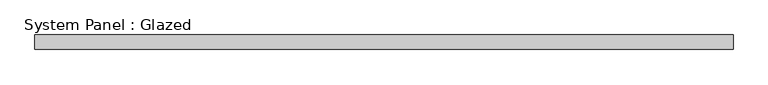
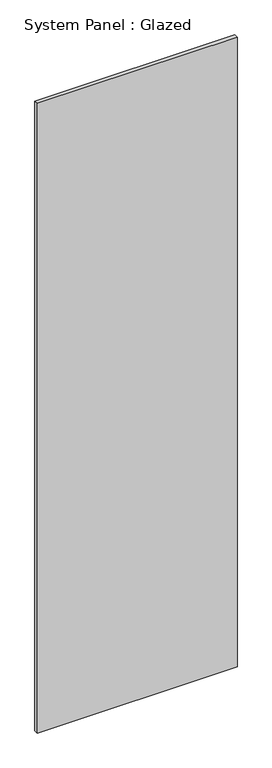
"""IFC4 building model written with IfcOpenShell, lengths in millimetres: plate geometry, System Panel : Glazed."""

from ifc_helpers import new_model, si_unit, origin, origin_with_axes, place, context, project, spatial, polyline, outline, extrude, source, transform, mapped, element, save


def system_panel_glazed_3e513c0f(model_context):
    return source(origin(), model_context, "Body", "SweptSolid", [
        extrude(outline(polyline([(600.1004, 24.5), (-600.1004, 24.5), (-600.1004, 49.5), (600.1004, 49.5), (600.1004, 24.5)])), origin_with_axes(), (0.0, 0.0, 1.0), 4000.0),
    ])


if __name__ == "__main__":
    model = new_model("IFC4")
    model_context = context("Model", 3, world=origin())
    ifc_project = project(units=[si_unit("LENGTHUNIT", "METRE", prefix="MILLI")], contexts=[model_context])
    site = spatial("IfcSite", under=ifc_project)
    building = spatial("IfcBuilding", under=site)
    placement = place(None, origin())
    system_panel_glazed_shape = system_panel_glazed_3e513c0f(model_context)
    element("IfcPlate", 1, ObjectType="System Panel : Glazed", at=placement, inside=building, context=model_context, shape_type="MappedRepresentation", body=[
        mapped(system_panel_glazed_shape, transform((0.0, 0.0, 0.0), x_axis=(1.0, 0.0, 0.0), y_axis=(0.0, 1.0, 0.0), z_axis=(0.0, 0.0, 1.0))),
    ])
    save(model, "model.ifc")

# Revit data of these elements
# Type "System Panel : Glazed"
#   Keynote = "H11"
#   Construction Type Id = "GSP4R"
#   Analytic Construction = "1/8 in Pilkington single glazing"
#   Visual Light Transmittance = 0.9
#   Solar Heat Gain Coefficient = 0.86
#   Heat Transfer Coefficient (U) = 6.7069 W/(m²·K)
#   Define Thermal Properties by = 1
# Element 1 (IfcPlate, "System Panel : Glazed")
#   Materials on its faces: "Glass"
# Materials
#   "Glass": class "Glass", colour RGB 0 128 192, transparency 0.9, Description = "Soda Lime Glass", Cost = 0
